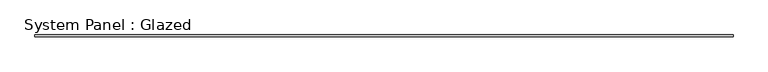
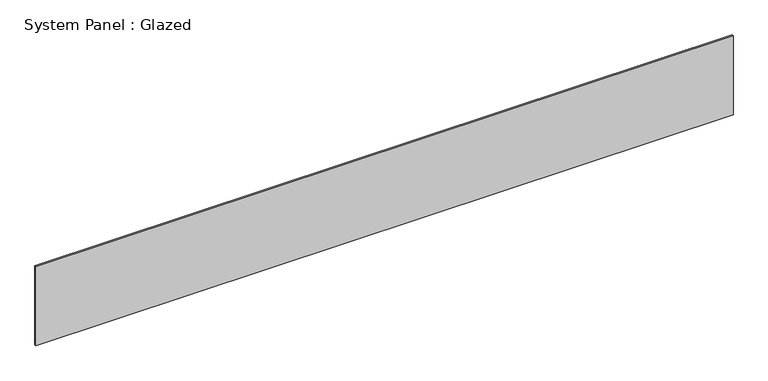
"""IFC4 building model written with IfcOpenShell, lengths in millimetres: plate geometry, System Panel : Glazed."""

from ifc_helpers import new_model, si_unit, origin, origin_with_axes, place, context, project, spatial, polyline, outline, extrude, source, transform, mapped, element, save


def system_panel_glazed_019fba88(model_context):
    return source(origin(), model_context, "Body", "SweptSolid", [
        extrude(outline(polyline([(5095.875, 19.05), (-5095.875, 19.05), (-5095.875, 44.45), (5095.875, 44.45), (5095.875, 19.05)])), origin_with_axes(), (0.0, 0.0, 1.0), 1219.2),
    ])


if __name__ == "__main__":
    model = new_model("IFC4")
    model_context = context("Model", 3, world=origin())
    ifc_project = project(units=[si_unit("LENGTHUNIT", "METRE", prefix="MILLI")], contexts=[model_context])
    site = spatial("IfcSite", under=ifc_project)
    building = spatial("IfcBuilding", under=site)
    placement = place(None, origin())
    system_panel_glazed_shape = system_panel_glazed_019fba88(model_context)
    element("IfcPlate", 1, ObjectType="System Panel : Glazed", at=placement, inside=building, context=model_context, shape_type="MappedRepresentation", body=[
        mapped(system_panel_glazed_shape, transform((0.0, 0.0, 0.0), x_axis=(1.0, 0.0, 0.0), y_axis=(0.0, 1.0, 0.0), z_axis=(0.0, 0.0, 1.0))),
    ])
    save(model, "model.ifc")

# Revit data of these elements
# Type "System Panel : Glazed"
#   Construction Type Id = "GSP4R"
#   Analytic Construction = "1/8 in Pilkington single glazing"
#   Visual Light Transmittance = 0.9
#   Solar Heat Gain Coefficient = 0.86
#   Heat Transfer Coefficient (U) = 1.18115 BTU/(h·ft²·°F)
# Element 1 (IfcPlate, "System Panel : Glazed")
#   Materials on its faces: "Glass"
# Materials
#   "Glass": class "Glass", colour RGB 0 128 192, transparency 0.75, Description = "Soda Lime Glass", Cost = 0
